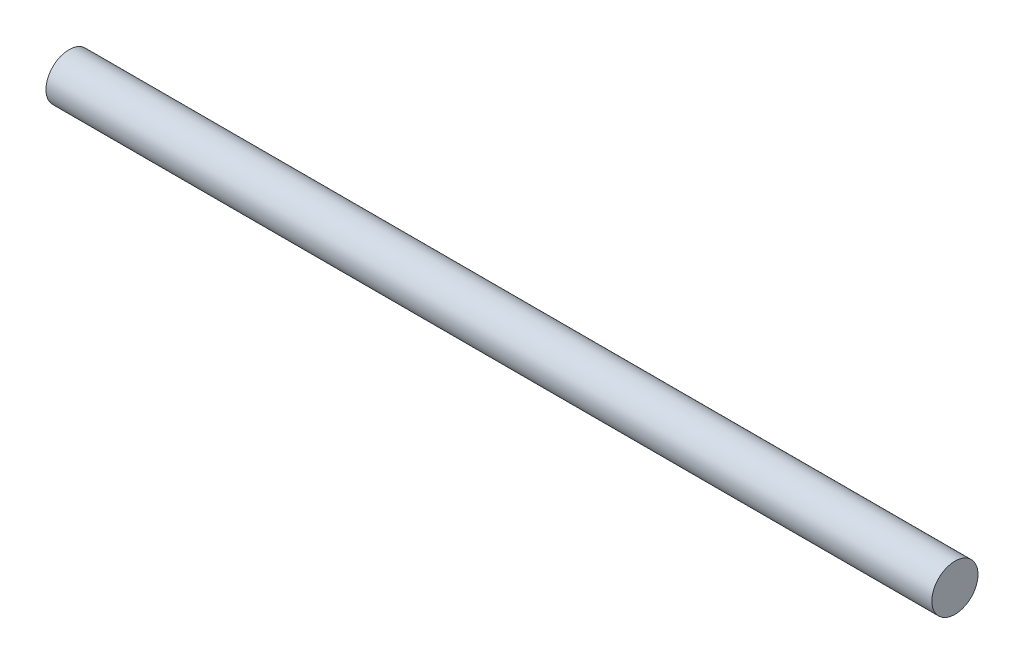
ISO-10303-21;
HEADER;
FILE_DESCRIPTION(('STEP AP214'),'2;1');
FILE_NAME('part.step','',(''),(''),'','','');
FILE_SCHEMA(('AUTOMOTIVE_DESIGN { 1 0 10303 214 1 1 1 1 }'));
ENDSEC;
DATA;
#1=APPLICATION_CONTEXT('core data for automotive mechanical design processes');
#2=APPLICATION_PROTOCOL_DEFINITION('international standard','automotive_design',2000,#1);
#3=PRODUCT_CONTEXT('',#1,'mechanical');
#4=PRODUCT('Part','Part','',(#3));
#5=PRODUCT_RELATED_PRODUCT_CATEGORY('part','',(#4));
#6=PRODUCT_DEFINITION_FORMATION('','',#4);
#7=PRODUCT_DEFINITION_CONTEXT('part definition',#1,'design');
#8=PRODUCT_DEFINITION('design','',#6,#7);
#9=PRODUCT_DEFINITION_SHAPE('','',#8);
#10=(LENGTH_UNIT() NAMED_UNIT(*) SI_UNIT(.MILLI.,.METRE.));
#11=(NAMED_UNIT(*) PLANE_ANGLE_UNIT() SI_UNIT($,.RADIAN.));
#12=(NAMED_UNIT(*) SI_UNIT($,.STERADIAN.) SOLID_ANGLE_UNIT());
#13=UNCERTAINTY_MEASURE_WITH_UNIT(LENGTH_MEASURE(1.E-05),#10,'distance_accuracy_value','');
#14=(GEOMETRIC_REPRESENTATION_CONTEXT(3) GLOBAL_UNCERTAINTY_ASSIGNED_CONTEXT((#13)) GLOBAL_UNIT_ASSIGNED_CONTEXT((#10,
#11,#12)) REPRESENTATION_CONTEXT('',''));
#15=CARTESIAN_POINT('',(0.,0.,0.));
#16=DIRECTION('',(0.,0.,1.));
#17=DIRECTION('',(1.,0.,0.));
#18=AXIS2_PLACEMENT_3D('',#15,#16,#17);
#19=CARTESIAN_POINT('',(96.,0.,0.));
#20=DIRECTION('',(-1.,0.,0.));
#21=DIRECTION('',(0.,0.,1.));
#22=AXIS2_PLACEMENT_3D('',#19,#20,#21);
#23=CYLINDRICAL_SURFACE('',#22,2.5);
#24=CARTESIAN_POINT('',(96.,0.,0.));
#25=DIRECTION('',(1.,0.,0.));
#26=DIRECTION('',(0.,0.,-1.));
#27=AXIS2_PLACEMENT_3D('',#24,#25,#26);
#28=CIRCLE('',#27,2.5);
#29=CARTESIAN_POINT('',(96.,0.,-2.5));
#30=VERTEX_POINT('',#29);
#31=EDGE_CURVE('E10',#30,#30,#28,.T.);
#32=ORIENTED_EDGE('',*,*,#31,.F.);
#33=EDGE_LOOP('',(#32));
#34=FACE_BOUND('',#33,.T.);
#35=CARTESIAN_POINT('',(0.,0.,0.));
#36=DIRECTION('',(1.,0.,0.));
#37=DIRECTION('',(0.,0.,-1.));
#38=AXIS2_PLACEMENT_3D('',#35,#36,#37);
#39=CIRCLE('',#38,2.5);
#40=CARTESIAN_POINT('',(0.,0.,-2.5));
#41=VERTEX_POINT('',#40);
#42=EDGE_CURVE('E45',#41,#41,#39,.T.);
#43=ORIENTED_EDGE('',*,*,#42,.T.);
#44=EDGE_LOOP('',(#43));
#45=FACE_BOUND('',#44,.T.);
#46=ADVANCED_FACE('F39',(#34,#45),#23,.T.);
#47=CARTESIAN_POINT('',(96.,0.,0.));
#48=DIRECTION('',(1.,0.,0.));
#49=DIRECTION('',(0.,0.,-1.));
#50=AXIS2_PLACEMENT_3D('',#47,#48,#49);
#51=PLANE('',#50);
#52=ORIENTED_EDGE('',*,*,#31,.T.);
#53=EDGE_LOOP('',(#52));
#54=FACE_BOUND('',#53,.T.);
#55=ADVANCED_FACE('F53',(#54),#51,.T.);
#56=CARTESIAN_POINT('',(0.,0.,0.));
#57=DIRECTION('',(1.,0.,0.));
#58=DIRECTION('',(0.,0.,-1.));
#59=AXIS2_PLACEMENT_3D('',#56,#57,#58);
#60=PLANE('',#59);
#61=ORIENTED_EDGE('',*,*,#42,.F.);
#62=EDGE_LOOP('',(#61));
#63=FACE_BOUND('',#62,.T.);
#64=ADVANCED_FACE('F55',(#63),#60,.F.);
#65=CLOSED_SHELL('',(#46,#55,#64));
#66=MANIFOLD_SOLID_BREP('B2',#65);
#67=ADVANCED_BREP_SHAPE_REPRESENTATION('',(#18,#66),#14);
#68=SHAPE_DEFINITION_REPRESENTATION(#9,#67);
ENDSEC;
END-ISO-10303-21;
